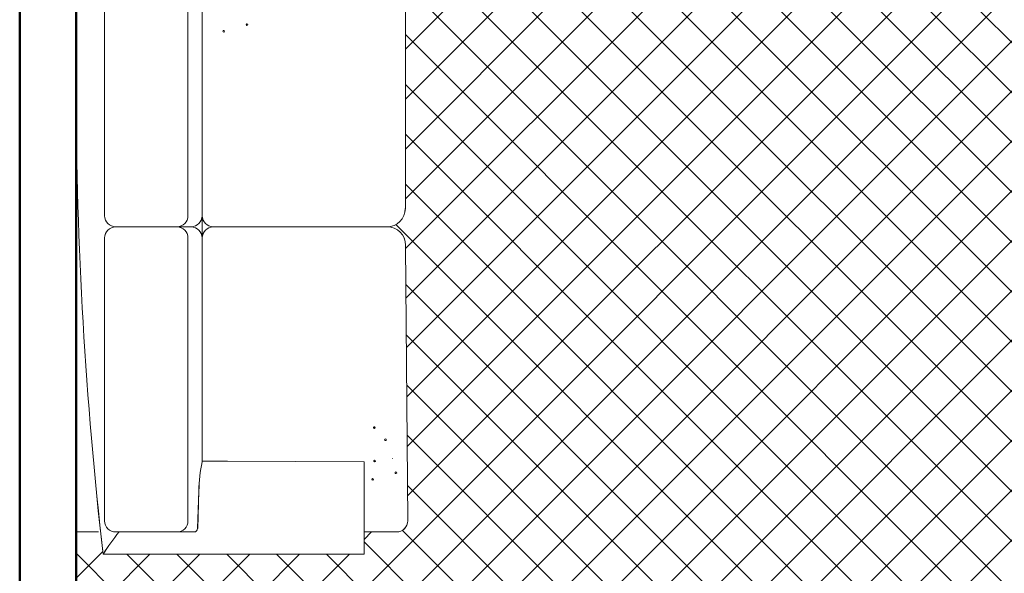
# Model space of a CAD drawing. Units: inches. Extents: x -466983 to 1020, y 324 to 318697.
# Tile 49 of 97: x 609 to 679, y 885 to 924. Entities that reach past the tile are written whole.
import ezdxf

# ---------------------------------------------------------------- set-up
doc = ezdxf.new("R2010")
doc.units = ezdxf.units.IN
doc.header["$MEASUREMENT"] = 0
for name, color, linetype, lineweight in [('A-FLOR-PATT', 252, 'Continuous', 13), ('A-FURN', 8, 'Continuous', 18), ('A-WALL', 7, 'Continuous', 50)]:
    doc.layers.add(name, color=color, linetype=linetype, lineweight=lineweight)

# ---------------------------------------------------------------- blocks, each defined once
blk = doc.blocks.new('L Shaped Sofa')
at = {"ltscale": 2}
for p, q in [((2438.01, 846.52), (2438.01, 834.58)), ((2471.77, 846.52), (2438.01, 846.52)), ((2438.01, 843.66), (2433.8, 843.66)), ((2459.54, 843.19), (2459.37, 838.32)), ((2460.02, 843.66), (2462.23, 843.66)), ((2470.14, 843.66), (2462.23, 843.66)), ((2475.26, 843.66), (2472.36, 843.66)), ((2475.26, 843.66), (2475.26, 821.69)), ((2432.65, 806.57), (2432.37, 842.21)), ((2460.8, 842.22), (2460.8, 821.69)), ((2471.57, 842.22), (2471.57, 821.69)), ((2455.69, 834.49), (2438.01, 834.58)), ((2455.69, 834.49), (2458.96, 834.49)), ((2458.96, 834.58), (2458.96, 805.64)), ((2460.8, 805.64), (2460.8, 821.69)), ((2471.57, 805.64), (2471.57, 821.69)), ((2475.26, 723.23), (2475.26, 821.69)), ((2458.96, 802.77), (2458.96, 805.64)), ((2435.07, 804.21), (2435.04, 804.21)), ((2457.53, 804.21), (2435.07, 804.21)), ((2457.53, 804.21), (2457.53, 804.21)), ((2462.23, 804.21), (2460.39, 804.21)), ((2470.14, 804.21), (2462.23, 804.21)), ((2458.96, 739.53), (2458.96, 802.77)), ((2460.8, 737.69), (2460.8, 802.77)), ((2471.57, 769.96), (2471.57, 802.77)), ((2432.68, 769.96), (2432.68, 801.82))]:
    blk.add_line(p, q, dxfattribs=at)
for centre, radius, start, end in [((2441.54, 866.11), 36.02, 321.4328, 327.0519), ((1939.08, 785.44), 536.19, 353.6823, 6.5416), ((2433.8, 842.22), 1.43, 90, 180.4579), ((2460.02, 843.18), 0.478, 90, 177.9816), ((2462.23, 842.22), 1.43, 90, 180), ((2470.14, 842.22), 1.43, 0, 90), ((2441.72, 838.37), 17.66, 347.6131, 359.8582), ((2436.91, 836.86), 0.106, 1.3946, 181.3946), ((2436.91, 836.86), 0.106, 181.3946, 1.3946), ((2433.9, 836), 0.106, 1.3946, 181.3946), ((2433.9, 836), 0.106, 181.3946, 1.3946), ((2434.34, 834.18), 0.0177, 1.3946, 181.3946), ((2434.34, 834.18), 0.0177, 181.3946, 1.3946), ((2436.66, 834.49), 0.106, 1.3946, 181.3946), ((2436.66, 834.49), 0.106, 181.3946, 1.3946), ((2435.25, 831.74), 0.106, 1.3946, 181.3946), ((2435.25, 831.74), 0.106, 181.3946, 1.3946), ((2436.69, 830.17), 0.106, 1.3946, 181.3946), ((2436.69, 830.17), 0.106, 181.3946, 1.3946), ((2435.04, 806.59), 2.39, 180.4579, 270), ((2457.53, 805.64), 1.43, 270, 0), ((2460.39, 805.64), 1.43, 180, 270), ((2462.23, 805.64), 1.43, 180, 270), ((2470.14, 805.64), 1.43, 270, 0), ((2435.07, 801.82), 2.39, 90, 180), ((2457.53, 802.77), 1.43, 0, 90), ((2460.39, 802.77), 1.43, 90, 180), ((2462.23, 802.77), 1.43, 90, 180), ((2470.14, 802.77), 1.43, 0, 90), ((2453.17, 778.06), 0.106, 1.3946, 181.3946), ((2456.17, 778.91), 0.106, 1.3946, 181.3946), ((2456.17, 778.91), 0.106, 181.3946, 1.3946), ((2453.17, 778.06), 0.106, 181.3946, 1.3946)]:
    blk.add_arc(centre, radius, start, end, dxfattribs=at)

msp = doc.modelspace()

# ---------------------------------------------------------------- hatches: boundary and pattern name
at = {"layer": 'A-FLOR-PATT', "transparency": 33554572}
h = msp.add_hatch(dxfattribs=at)
h.set_pattern_fill('ANSI37', color=256, scale=30)
h.set_pattern_definition([(45, (-1212.4137, -290.035), (-2.6516504, 2.6516504), []), (135, (-1212.4137, -290.035), (-2.6516504, -2.6516504), [])])
h.paths.add_polyline_path([(901.806, 1075.938), (900.614, 1075.938), (900.614, 1065.386), (899.391, 1065.386), (898.091, 1065.386), (892.836, 1058.71, -0.258377), (892.188, 1058.351), (879.985, 1058.351, -0.20177), (879.438, 1058.581), (874.081, 1065.386), (872.781, 1065.386), (871.558, 1065.386), (871.558, 1075.938), (813.806, 1075.938), (813.806, 1044.792), (832.395, 1044.792, -0.394795), (848.66, 1028.536), (848.66, 1009.938), (901.806, 1009.938), (901.806, 1015.938), (901.306, 1015.938), (871.306, 1015.938), (871.306, 1017.25), (871.334, 1017.25, -0.401453), (901.306, 1045.938), (901.806, 1045.938)])
edge = h.paths.add_edge_path(flags=16)
edge.add_line((847.773, 1068.949), (847.773, 1073.709))
edge.add_arc((849.227, 1073.709), 1.454, 90, 180, ccw=False)
edge.add_line((849.227, 1075.163), (864.492, 1075.163))
edge.add_arc((864.492, 1073.709), 1.454, 0, 90, ccw=False)
edge.add_line((865.946, 1073.709), (865.946, 1069.004))
edge.add_arc((832.645, 1068.976), 33.301, -20.61234, 0.04725, ccw=False)
edge.add_ellipse((856.859, 1058.48), major_axis=(0, 10.213), ratio=0.685919, start_angle=100.00884, end_angle=259.99116, ccw=False)
edge.add_arc((881.074, 1068.976), 33.301, 180.04725, 200.61234, ccw=False)
h.paths.add_polyline_path([(853.146, 1066.482), (853.146, 1066.453), (853.146, 1066.453, 0.433107), (852.917, 1066.685), (852.917, 1066.453), (853.146, 1066.453), (853.146, 1066.482), (853.088, 1066.612, 0.697939), (852.7, 1066.453), (852.7, 1066.453), (852.7, 1066.482), (852.917, 1067.001), (852.917, 1066.685, -0.396254)], flags=0)
h.paths.add_polyline_path([(861.019, 1066.482), (861.019, 1066.453), (861.019, 1066.453, 0.416404), (860.802, 1066.685), (860.802, 1066.453), (861.019, 1066.453), (861.019, 1066.482), (860.967, 1066.605, 0.713344), (860.573, 1066.453), (860.573, 1066.453), (860.573, 1066.482), (860.802, 1067.001), (860.802, 1066.685, -0.379973)], flags=0)
edge = h.paths.add_edge_path(flags=0)
edge.add_spline(control_points=[(861.13, 1065.785), (861.466, 1065.248), (861.613, 1065.016), (861.983, 1064.374), (862.192, 1063.944), (862.561, 1063.039), (862.721, 1062.563), (862.987, 1061.578), (863.092, 1061.069), (863.245, 1060.031), (863.293, 1059.503), (863.329, 1058.441), (863.318, 1057.908), (863.237, 1056.852), (863.166, 1056.329), (862.97, 1055.308), (862.843, 1054.81), (862.537, 1053.852), (862.357, 1053.393), (861.951, 1052.525), (861.725, 1052.117), (861.233, 1051.362), (860.967, 1051.016), (860.405, 1050.395), (860.108, 1050.12), (859.494, 1049.646), (859.176, 1049.448), (858.528, 1049.13), (858.197, 1049.011), (857.531, 1048.852), (857.196, 1048.812), (856.525, 1048.812), (856.189, 1048.852), (855.524, 1049.01), (855.193, 1049.129), (854.545, 1049.447), (854.227, 1049.645), (853.612, 1050.118), (853.316, 1050.393), (852.753, 1051.014), (852.487, 1051.36), (851.995, 1052.114), (851.769, 1052.523), (851.363, 1053.39), (851.183, 1053.85), (850.877, 1054.807), (850.75, 1055.305), (850.553, 1056.326), (850.483, 1056.849), (850.401, 1057.905), (850.39, 1058.438), (850.426, 1059.5), (850.473, 1060.028), (850.626, 1061.066), (850.732, 1061.575), (850.997, 1062.561), (851.157, 1063.036), (851.525, 1063.942), (851.734, 1064.371), (852.106, 1065.016), (852.254, 1065.25), (852.608, 1065.733)], knot_values=[3.915332, 3.915332, 3.915332, 3.915332, 4.013468, 4.013468, 4.175532, 4.175532, 4.337596, 4.337596, 4.49966, 4.49966, 4.661724, 4.661724, 4.823788, 4.823788, 4.985852, 4.985852, 5.147916, 5.147916, 5.30998, 5.30998, 5.472044, 5.472044, 5.634109, 5.634109, 5.796173, 5.796173, 5.958237, 5.958237, 6.120301, 6.120301, 6.282365, 6.282365, 6.444429, 6.444429, 6.606493, 6.606493, 6.768557, 6.768557, 6.930621, 6.930621, 7.092685, 7.092685, 7.254749, 7.254749, 7.416813, 7.416813, 7.578878, 7.578878, 7.740942, 7.740942, 7.903006, 7.903006, 8.06507, 8.06507, 8.227134, 8.227134, 8.389198, 8.389198, 8.551262, 8.551262, 8.65037, 8.65037, 8.65037, 8.65037], degree=3, periodic=0)
edge.add_line((852.642, 1065.785), (861.13, 1065.785))
edge = h.paths.add_edge_path(flags=0)
edge.add_ellipse((856.85, 1057.743), major_axis=(0, 7.792), ratio=0.687861, start_angle=0, end_angle=360)
h.paths.add_polyline_path([(848.863, 1069.389), (848.863, 1073.96, -0.414214), (849.954, 1075.051), (863.765, 1075.051, -0.414214), (864.856, 1073.96), (864.856, 1069.389, -0.388936), (864.524, 1069.027, -0.043561), (849.195, 1069.027, -0.388936)], flags=0)
h.paths.add_polyline_path([(853.101, 1068.112, -1), (852.677, 1068.112, -1)], flags=0)
edge = h.paths.add_edge_path(flags=0)
edge.add_ellipse((856.859, 1057.338), major_axis=(0, 2.207), ratio=0.657164, start_angle=0, end_angle=360)
h.paths.add_polyline_path([(861.041, 1068.112, -1), (860.618, 1068.112, -1)], flags=0)
edge = h.paths.add_edge_path()
edge.add_line((573.954, 1057.341), (573.954, 1075.938))
edge.add_line((573.954, 1075.938), (558.731, 1075.938))
edge.add_line((558.731, 1075.938), (558.731, 1065.386))
edge.add_line((558.731, 1065.386), (557.507, 1065.386))
edge.add_line((557.507, 1065.386), (556.207, 1065.386))
edge.add_line((556.207, 1065.386), (550.952, 1058.71))
edge.add_arc((550.304, 1059.116), 0.765, 270, 327.94832, ccw=False)
edge.add_line((550.304, 1058.351), (538.101, 1058.351))
edge.add_arc((538.101, 1059.116), 0.765, 224.3704, 270, ccw=False)
edge.add_line((537.555, 1058.581), (532.198, 1065.386))
edge.add_line((532.198, 1065.386), (530.898, 1065.386))
edge.add_line((530.898, 1065.386), (529.674, 1065.386))
edge.add_line((529.674, 1065.386), (529.674, 1075.938))
edge.add_line((529.674, 1075.938), (520.806, 1075.938))
edge.add_line((520.806, 1075.938), (520.806, 1045.938))
edge.add_line((520.806, 1045.938), (521.306, 1045.938))
edge.add_arc((521.306, 1015.938), 30, 2.50749, 90, ccw=False)
edge.add_line((551.277, 1017.25), (551.306, 1017.25))
edge.add_line((551.306, 1017.25), (551.306, 1015.938))
edge.add_line((551.306, 1015.938), (520.806, 1015.938))
edge.add_line((520.806, 1015.938), (520.806, 1009.938))
edge.add_line((520.806, 1009.938), (559.191, 1010.402))
edge.add_arc((559.191, 1011.856), 1.454, 180, 270, ccw=False)
edge.add_line((557.737, 1011.856), (557.737, 1016.561))
edge.add_arc((591.039, 1016.589), 33.301, 159.38766, 180.04725, ccw=False)
edge.add_ellipse((566.824, 1027.085), major_axis=(0, 10.213), ratio=0.685919, start_angle=280.00884, end_angle=439.99116, ccw=False)
edge.add_arc((542.609, 1016.589), 33.301, 0.04725, 20.61234, ccw=False)
edge.add_line((575.91, 1016.616), (575.91, 1011.856))
edge.add_arc((574.456, 1011.856), 1.454, -90, 0, ccw=False)
edge.add_line((574.456, 1010.402), (608.806, 1009.938))
edge.add_line((608.806, 1009.938), (608.806, 1041.086))
edge.add_line((608.806, 1041.086), (590.218, 1041.086))
edge.add_arc((590.775, 1057.907), 16.831, 181.92775, 268.10321, ccw=False)
edge = h.paths.add_edge_path()
edge.add_ellipse((494.244, 583.62), major_axis=(0, 10.213), ratio=0.685919, start_angle=280.00884, end_angle=439.99116, ccw=False)
edge.add_arc((470.03, 573.124), 33.301, 0.04725, 20.61234, ccw=False)
edge.add_line((503.331, 573.152), (503.331, 568.392))
edge.add_arc((501.877, 568.392), 1.454, -90, 0, ccw=False)
edge.add_line((501.877, 566.938), (539.806, 566.938))
edge.add_line((539.806, 566.938), (539.806, 572.938))
edge.add_line((539.806, 572.938), (539.306, 572.938))
edge.add_line((539.306, 572.938), (509.306, 572.938))
edge.add_line((509.306, 572.938), (509.306, 574.25))
edge.add_line((509.306, 574.25), (509.334, 574.25))
edge.add_arc((539.306, 572.938), 30, 90, 177.49251, ccw=False)
edge.add_line((539.306, 602.938), (539.806, 602.938))
edge.add_line((539.806, 602.938), (539.806, 626.938))
edge.add_line((539.806, 626.938), (531.772, 626.938))
edge.add_line((531.772, 626.938), (531.772, 616.386))
edge.add_line((531.772, 616.386), (530.548, 616.386))
edge.add_line((530.548, 616.386), (529.249, 616.386))
edge.add_line((529.249, 616.386), (523.711, 609.351))
edge.add_line((523.711, 609.351), (510.777, 609.351))
edge.add_line((510.777, 609.351), (505.239, 616.386))
edge.add_line((505.239, 616.386), (503.939, 616.386))
edge.add_line((503.939, 616.386), (502.715, 616.386))
edge.add_line((502.715, 616.386), (502.715, 626.938))
edge.add_line((502.715, 626.938), (481.698, 626.938))
edge.add_line((481.698, 626.938), (481.698, 610.995))
edge.add_arc((467.27, 611.473), 14.436, 271.92775, 358.10321, ccw=False)
edge.add_line((467.756, 597.045), (451.806, 597.045))
edge.add_line((451.806, 597.045), (451.806, 584.404))
edge.add_line((451.806, 584.404), (451.806, 566.938))
edge.add_line((451.806, 566.938), (486.612, 566.938))
edge.add_arc((486.612, 568.392), 1.454, 180, 270, ccw=False)
edge.add_line((485.158, 568.392), (485.158, 573.097))
edge.add_arc((518.459, 573.124), 33.301, 159.38766, 180.04725, ccw=False)
h.paths.add_polyline_path([(836.261, 1020.733), (879.89, 1020.733), (879.89, 1039.39), (836.261, 1039.39)], flags=25)
h.paths.add_polyline_path([(549.985, 1036.749), (593.614, 1036.749), (593.614, 1055.407), (549.985, 1055.407)], flags=24)
h.paths.add_polyline_path([(475.123, 595.596), (518.752, 595.596), (518.752, 614.253), (475.123, 614.253)], flags=24)
h = msp.add_hatch(dxfattribs=at)
h.set_pattern_fill('ANSI37', color=256, scale=20)
h.set_pattern_definition([(45, (-1212.4137, -290.035), (-1.767767, 1.767767), []), (135, (-1212.4137, -290.035), (-1.767767, -1.767767), [])])
h.paths.add_polyline_path([(809.806, 870.938), (809.806, 888.152), (806.998, 888.152), (802.662, 888.152), (789.383, 888.152), (786.285, 888.152, -0.414214), (785.499, 888.937), (785.499, 900.196), (785.499, 908.47, -0.414214), (786.808, 909.779, -0.414214), (785.499, 911.088), (785.499, 929.101, -0.414214), (786.808, 930.411, -0.414214), (785.499, 931.72), (785.499, 931.904, -0.414214), (784.19, 930.595), (766.722, 930.595, -0.412359), (765.413, 931.896, -0.413741), (764.115, 930.578), (744.578, 930.422, -0.416556), (743.786, 931.207), (743.786, 933.515), (742.215, 933.515), (742.215, 952.024, -0.001344), (743.786, 952.2), (743.786, 953.938), (678.592, 953.938), (678.592, 951.131), (678.592, 946.794), (678.592, 933.515), (678.592, 930.417, -0.414214), (677.806, 929.631), (666.548, 929.631), (658.274, 929.631, -0.414214), (656.965, 930.94, -0.414214), (655.656, 929.631), (637.642, 929.631, -0.414214), (636.333, 930.94, -0.414214), (635.024, 929.631), (634.839, 929.631, -0.414214), (636.149, 928.322), (636.149, 910.854, -0.412359), (634.848, 909.545, -0.413741), (636.165, 908.247), (636.321, 888.71, -0.416556), (635.536, 887.918), (633.228, 887.918), (633.228, 886.347), (614.719, 886.347, -0.001344), (614.544, 887.918), (612.806, 887.918), (612.806, 834.938), (612.806, 752.938), (612.806, 748.938), (612.806, 697.938), (654.806, 697.938), (654.806, 701.938), (715.806, 701.938), (715.806, 737.435), (774.292, 737.435), (774.292, 795.938), (809.806, 795.938)])
h.paths.add_polyline_path([(679.276, 849.576, 0.102523), (682.148, 849.261, -0.080461), (694.543, 849.773, -0.283899), (694.482, 849.008, 0.136605), (694.407, 848.81, -0.030441), (694.543, 846.893), (694.543, 842.62), (694.543, 838.347, -0.028219), (694.425, 836.568), (694.425, 836.568, 0.196187), (694.446, 836.271, -0.302897), (694.543, 835.467, -0.080461), (682.148, 835.979, 0.102523), (679.276, 835.664, -0.58611), (678.646, 836.017), (678.646, 849.223, -0.58611)], flags=16)
h.paths.add_polyline_path([(679.517, 848.651, 0.699597), (679.476, 848.634, 1.20716), (679.194, 848.742, 0.010621)], flags=0)
h.paths.add_polyline_path([(679.492, 836.561, -0.013798), (679.918, 836.659, -0.071703), (682.853, 837.143, -0.165743), (682.166, 839.101), (682.166, 842.609), (682.166, 846.06, -0.240616), (683.473, 848.677, -0.068263), (693.929, 849.008), (693.788, 848.708), (693.788, 849.023, 0.067332), (683.473, 848.677, 0.240616), (682.166, 846.06), (682.166, 842.609), (682.166, 839.101, 0.23459), (683.461, 836.551, 0.068093), (693.788, 836.195), (693.788, 836.51), (693.93, 836.21, -0.077215), (682.242, 836.782, 0.086627), (679.528, 836.57, -0.628402), (679.503, 836.573), (679.503, 836.607, 0.910458)], flags=0)
h.paths.add_polyline_path([(679.476, 848.636), (679.207, 848.647), (679.207, 836.572, 0.913566), (679.365, 836.586), (679.476, 836.582)], flags=0)
h.paths.add_polyline_path([(679.276, 829.86, 0.102523), (682.148, 829.546, -0.080461), (694.543, 830.057, -0.283899), (694.482, 829.293, 0.136605), (694.407, 829.095, -0.030441), (694.543, 827.178), (694.543, 822.904), (694.543, 818.631, -0.028219), (694.425, 816.853), (694.425, 816.853, 0.196187), (694.446, 816.556, -0.302897), (694.543, 815.752, -0.080461), (682.148, 816.263, 0.102523), (679.276, 815.949, -0.58611), (678.646, 816.302), (678.646, 829.507, -0.58611)], flags=16)
h.paths.add_polyline_path([(679.517, 828.936, 0.699597), (679.476, 828.919, 1.20716), (679.194, 829.027, 0.010621)], flags=0)
h.paths.add_polyline_path([(679.492, 816.846, -0.013798), (679.918, 816.944, -0.071703), (682.853, 817.428, -0.165743), (682.166, 819.385), (682.166, 822.894), (682.166, 826.345, -0.240616), (683.473, 828.961, -0.068263), (693.929, 829.293), (693.788, 828.993), (693.788, 829.308, 0.067332), (683.473, 828.961, 0.240616), (682.166, 826.345), (682.166, 822.894), (682.166, 819.385, 0.23459), (683.461, 816.836, 0.068093), (693.788, 816.48), (693.788, 816.795), (693.93, 816.495, -0.077215), (682.242, 817.066, 0.086627), (679.528, 816.855, -0.628402), (679.503, 816.858), (679.503, 816.892, 0.910458)], flags=0)
h.paths.add_polyline_path([(679.476, 828.921), (679.207, 828.932), (679.207, 816.857, 0.913566), (679.365, 816.871), (679.476, 816.867)], flags=0)
h.paths.add_polyline_path([(679.276, 810.145, 0.102523), (682.148, 809.83, -0.080461), (694.543, 810.342, -0.3023), (694.447, 809.539, 0.10023), (694.406, 809.388, -0.03057), (694.543, 807.462), (694.543, 803.189), (694.543, 798.916, -0.03057), (694.406, 796.991, 0.10023), (694.447, 796.839, -0.3023), (694.543, 796.036, -0.080461), (682.148, 796.548, 0.102523), (679.276, 796.233, -0.58611), (678.646, 796.586), (678.646, 809.792, -0.58611)], flags=16)
h.paths.add_polyline_path([(679.517, 809.242, 0.699597), (679.476, 809.224, 1.20716), (679.194, 809.332, 0.010621)], flags=0)
h.paths.add_polyline_path([(679.492, 797.151, -0.013798), (679.918, 797.25, -0.071703), (682.853, 797.734, -0.165743), (682.166, 799.691), (682.166, 803.2), (682.166, 806.65, -0.239349), (683.461, 809.258, -0.072465), (694.447, 809.541, 0.197932), (694.425, 809.241), (693.788, 809.299), (693.788, 809.614, 0.068093), (683.461, 809.258, 0.239349), (682.166, 806.65), (682.166, 803.2), (682.166, 799.691, 0.235854), (683.473, 797.132, 0.067332), (693.788, 796.786), (693.788, 797.101), (694.425, 797.159, 0.197932), (694.447, 796.859, -0.080419), (682.156, 797.379, 0.083867), (679.528, 797.16, -0.628402), (679.503, 797.164), (679.503, 797.197, 0.910458)], flags=0)
h.paths.add_polyline_path([(679.207, 809.237), (679.207, 797.162, 0.913566), (679.365, 797.176), (679.476, 797.173), (679.476, 809.227)], flags=0)
h.paths.add_polyline_path([(695.364, 853.299), (728.223, 853.299), (728.223, 771.152), (695.364, 771.152)], flags=16)
h.paths.add_polyline_path([(696.021, 852.642), (727.566, 852.642), (727.566, 771.809), (696.021, 771.809)], flags=0)
h.paths.add_polyline_path([(679.276, 788.787, 0.102523), (682.148, 788.472, -0.080461), (694.543, 788.984, -0.3023), (694.447, 788.181, 0.10023), (694.406, 788.03, -0.03057), (694.543, 786.104), (694.543, 781.831), (694.543, 777.558, -0.03057), (694.406, 775.632, 0.10023), (694.447, 775.481, -0.3023), (694.543, 774.678, -0.080461), (682.148, 775.19, 0.102523), (679.276, 774.875, -0.58611), (678.646, 775.228), (678.646, 788.434, -0.58611)], flags=16)
h.paths.add_polyline_path([(679.517, 787.883, 0.699597), (679.476, 787.866, 1.20716), (679.194, 787.974, 0.010621)], flags=0)
h.paths.add_polyline_path([(679.492, 775.793, -0.013798), (679.918, 775.891, -0.071703), (682.853, 776.375, -0.165743), (682.166, 778.333), (682.166, 781.841), (682.166, 785.292, -0.239349), (683.461, 787.899, -0.072465), (694.447, 788.182, 0.197932), (694.425, 787.882), (693.788, 787.94), (693.788, 788.255, 0.068093), (683.461, 787.899, 0.239349), (682.166, 785.292), (682.166, 781.841), (682.166, 778.333, 0.235854), (683.473, 775.774, 0.067332), (693.788, 775.428), (693.788, 775.742), (694.425, 775.8, 0.197932), (694.447, 775.5, -0.080419), (682.156, 776.021, 0.083867), (679.528, 775.802, -0.628402), (679.503, 775.805), (679.503, 775.839, 0.910458)], flags=0)
h.paths.add_polyline_path([(679.207, 787.879), (679.207, 775.804, 0.913566), (679.365, 775.818), (679.476, 775.814), (679.476, 787.868)], flags=0)
h.paths.add_polyline_path([(704.641, 854.12, -0.080461), (705.153, 866.516, 0.102523), (704.838, 869.387, -0.58611), (705.191, 870.017), (718.397, 870.017, -0.58611), (718.75, 869.387, 0.102523), (718.435, 866.516, -0.080461), (718.946, 854.12, -0.3023), (718.144, 854.217, 0.10023), (717.992, 854.257, -0.03057), (716.067, 854.12), (711.794, 854.12), (707.521, 854.12, -0.03057), (705.595, 854.257, 0.10023), (705.444, 854.217, -0.3023)], flags=16)
h.paths.add_polyline_path([(717.846, 869.146, 0.699597), (717.829, 869.187, 1.20716), (717.937, 869.47, 0.010621)], flags=0)
h.paths.add_polyline_path([(705.463, 854.216, -0.080419), (705.984, 866.507, 0.083867), (705.765, 869.135, -0.628402), (705.768, 869.16), (705.802, 869.16, 0.910458), (705.756, 869.171, -0.013798), (705.854, 868.745, -0.071703), (706.338, 865.81, -0.165743), (708.295, 866.497), (711.804, 866.497), (715.255, 866.497, -0.239349), (717.862, 865.202, -0.072465), (718.145, 854.216, 0.197932), (717.845, 854.238), (717.903, 854.876), (718.218, 854.876, 0.068093), (717.862, 865.202, 0.239349), (715.255, 866.497), (711.804, 866.497), (708.295, 866.497, 0.235854), (705.737, 865.19, 0.067332), (705.391, 854.876), (705.705, 854.876), (705.763, 854.238, 0.197932)], flags=16)
h.paths.add_polyline_path([(705.766, 869.456, 0.913566), (705.781, 869.299), (705.777, 869.187), (717.831, 869.187), (717.842, 869.456)], flags=0)
h.paths.add_polyline_path([(729.045, 842.62), (729.045, 846.893, -0.03057), (729.182, 848.818, 0.10023), (729.141, 848.97, -0.3023), (729.045, 849.773, -0.080461), (741.44, 849.261, 0.102523), (744.311, 849.576, -0.58611), (744.942, 849.223), (744.942, 836.017, -0.58611), (744.311, 835.664, 0.102523), (741.44, 835.979, -0.080461), (729.045, 835.467, -0.3023), (729.141, 836.27, 0.10023), (729.182, 836.421, -0.03057), (729.045, 838.347)], flags=16)
h.paths.add_polyline_path([(744.111, 836.585, 1.20716), (744.394, 836.477, 0.010621), (744.07, 836.567, 0.699597)], flags=0)
h.paths.add_polyline_path([(729.141, 836.268, 0.197932), (729.162, 836.568), (729.8, 836.51), (729.8, 836.195, 0.068093), (740.126, 836.551, 0.239349), (741.421, 839.159), (741.421, 842.609), (741.421, 846.118, 0.235854), (740.114, 848.677, 0.067332), (729.8, 849.023), (729.8, 848.708), (729.162, 848.65, 0.197932), (729.141, 848.95, -0.080419), (741.432, 848.43, 0.083867), (744.059, 848.649, -0.628402), (744.085, 848.645), (744.085, 848.612, 0.910458), (744.095, 848.658, -0.013798), (743.67, 848.559, -0.071703), (740.734, 848.075, -0.165743), (741.421, 846.118), (741.421, 842.609), (741.421, 839.159, -0.239349), (740.126, 836.551, -0.072465)], flags=0)
h.paths.add_polyline_path([(729.045, 830.057, -0.080461), (741.44, 829.546, 0.102523), (744.311, 829.86, -0.58611), (744.942, 829.507), (744.942, 816.302, -0.58611), (744.311, 815.949, 0.102523), (741.44, 816.263, -0.080461), (729.045, 815.752, -0.3023), (729.141, 816.554, 0.10023), (729.182, 816.706, -0.03057), (729.045, 818.631), (729.045, 822.904), (729.045, 827.178, -0.03057), (729.182, 829.103, 0.10023), (729.141, 829.255, -0.3023)], flags=16)
h.paths.add_polyline_path([(744.111, 816.869, 1.20716), (744.394, 816.761, 0.010621), (744.07, 816.852, 0.699597)], flags=0)
h.paths.add_polyline_path([(729.141, 829.235, -0.080419), (741.432, 828.714, 0.083867), (744.059, 828.933, -0.628402), (744.085, 828.93), (744.085, 828.896, 0.910458), (744.095, 828.943, -0.013798), (743.67, 828.844, -0.071703), (740.734, 828.36, -0.165743), (741.421, 826.403), (741.421, 822.894), (741.421, 819.443, -0.239349), (740.126, 816.836, -0.072465), (729.141, 816.553, 0.197932), (729.162, 816.853), (729.8, 816.795), (729.8, 816.48, 0.068093), (740.126, 816.836, 0.239349), (741.421, 819.443), (741.421, 822.894), (741.421, 826.403, 0.235854), (740.114, 828.961, 0.067332), (729.8, 829.308), (729.8, 828.993), (729.162, 828.935, 0.197932)], flags=16)
h.paths.add_polyline_path([(729.045, 810.342, -0.080461), (741.44, 809.83, 0.102523), (744.311, 810.145, -0.58611), (744.942, 809.792), (744.942, 796.586, -0.58611), (744.311, 796.233, 0.102523), (741.44, 796.548, -0.080461), (729.045, 796.036, -0.283899), (729.105, 796.801, 0.136605), (729.181, 796.999, -0.030441), (729.045, 798.916), (729.045, 803.189), (729.045, 807.462, -0.028219), (729.163, 809.241), (729.162, 809.241, 0.196187), (729.142, 809.538, -0.302897)], flags=16)
h.paths.add_polyline_path([(744.111, 797.175, 1.20716), (744.394, 797.067, 0.010621), (744.07, 797.158, 0.699597)], flags=0)
h.paths.add_polyline_path([(741.345, 809.027, 0.086627), (744.059, 809.239, -0.628402), (744.085, 809.235), (744.085, 809.202, 0.910458), (744.095, 809.248, -0.013798), (743.67, 809.15, -0.071703), (740.734, 808.666, -0.165743), (741.421, 806.708), (741.421, 803.2), (741.421, 799.749, -0.240616), (740.114, 797.132, -0.068263), (729.658, 796.801), (729.8, 797.101), (729.8, 796.786, 0.067332), (740.114, 797.132, 0.240616), (741.421, 799.749), (741.421, 803.2), (741.421, 806.708, 0.23459), (740.126, 809.258, 0.068093), (729.8, 809.614), (729.8, 809.299), (729.658, 809.599, -0.077215)], flags=0)
h.paths.add_polyline_path([(704.641, 770.33, -0.283899), (705.405, 770.27, 0.136605), (705.603, 770.194, -0.030441), (707.521, 770.33), (711.794, 770.33), (716.067, 770.33, -0.028219), (717.845, 770.212), (717.845, 770.213, 0.196187), (718.143, 770.233, -0.302897), (718.946, 770.33, -0.080461), (718.435, 757.935, 0.102523), (718.75, 755.064, -0.58611), (718.397, 754.433), (705.191, 754.433, -0.58611), (704.838, 755.064, 0.102523), (705.153, 757.935, -0.080461)], flags=16)
h.paths.add_polyline_path([(705.762, 755.305, 0.699597), (705.779, 755.264, 1.20716), (705.671, 754.981, 0.010621)], flags=0)
h.paths.add_polyline_path([(705.405, 769.717), (705.705, 769.575), (705.391, 769.575, 0.067332), (705.737, 759.261, 0.240616), (708.353, 757.954), (711.804, 757.954), (715.313, 757.954, 0.23459), (717.862, 759.249, 0.068093), (718.218, 769.575), (717.903, 769.575), (718.203, 769.717, -0.077215), (717.632, 758.03, 0.086627), (717.843, 755.316, -0.628402), (717.84, 755.29), (717.806, 755.29, 0.910458), (717.853, 755.28, -0.013798), (717.754, 755.705, -0.071703), (717.27, 758.641, -0.165743), (715.313, 757.954), (711.804, 757.954), (708.353, 757.954, -0.240616), (705.737, 759.261, -0.068263)], flags=0)
h.paths.add_polyline_path([(729.045, 788.984, -0.080461), (741.44, 788.472, 0.102523), (744.311, 788.787, -0.58611), (744.942, 788.434), (744.942, 775.228, -0.58611), (744.311, 774.875, 0.102523), (741.44, 775.19, -0.080461), (729.045, 774.678, -0.283899), (729.105, 775.443, 0.136605), (729.181, 775.64, -0.030441), (729.045, 777.558), (729.045, 781.831), (729.045, 786.104, -0.028219), (729.163, 787.882), (729.162, 787.882, 0.196187), (729.142, 788.18, -0.302897)], flags=16)
h.paths.add_polyline_path([(744.111, 775.817, 1.20716), (744.394, 775.709, 0.010621), (744.07, 775.799, 0.699597)], flags=0)
h.paths.add_polyline_path([(741.345, 787.669, 0.086627), (744.059, 787.881, -0.628402), (744.085, 787.877), (744.085, 787.844, 0.910458), (744.095, 787.89, -0.013798), (743.67, 787.791, -0.071703), (740.734, 787.307, -0.165743), (741.421, 785.35), (741.421, 781.841), (741.421, 778.39, -0.240616), (740.114, 775.774, -0.068263), (729.658, 775.443), (729.8, 775.742), (729.8, 775.428, 0.067332), (740.114, 775.774, 0.240616), (741.421, 778.39), (741.421, 781.841), (741.421, 785.35, 0.23459), (740.126, 787.899, 0.068093), (729.8, 788.255), (729.8, 787.94), (729.658, 788.241, -0.077215)], flags=0)
h.paths.add_polyline_path([(744.111, 848.636), (744.111, 836.582), (744.381, 836.572), (744.381, 848.647, 0.913566), (744.223, 848.633)], flags=0)
h.paths.add_polyline_path([(744.223, 828.917), (744.111, 828.921), (744.111, 816.867), (744.381, 816.857), (744.381, 828.932, 0.913566)], flags=0)
h.paths.add_polyline_path([(717.831, 755.264), (705.777, 755.264), (705.766, 754.994), (717.842, 754.994, 0.913566), (717.827, 755.152)], flags=0)
h.paths.add_polyline_path([(744.223, 809.223), (744.111, 809.227), (744.111, 797.173), (744.381, 797.162), (744.381, 809.237, 0.913566)], flags=0)
h.paths.add_polyline_path([(744.111, 787.868), (744.111, 775.814), (744.381, 775.804), (744.381, 787.879, 0.913566), (744.223, 787.865)], flags=0)
h.paths.add_polyline_path([(678.877, 877.123), (737.613, 877.123), (737.613, 899.512), (678.877, 899.512)], flags=24)

# ---------------------------------------------------------------- linework, layer by layer
at = {"layer": 'A-FURN', "ltscale": 2}
for p, q in [((612.806, 953.938), (612.806, 899.962)), ((612.806, 953.938), (612.806, 899.962)), ((612.806, 953.938), (612.806, 899.962)), ((612.806, 953.938), (612.806, 899.962)), ((612.806, 953.938), (612.806, 899.962)), ((612.806, 953.938), (612.806, 899.962)), ((620.734, 946.009), (620.734, 910.331)), ((620.734, 946.009), (620.734, 910.331)), ((620.734, 946.009), (620.734, 910.331)), ((620.734, 946.009), (620.734, 910.331)), ((620.734, 946.009), (620.734, 910.331)), ((620.734, 946.009), (620.734, 910.331)), ((621.743, 945), (621.743, 910.331)), ((621.743, 945), (621.743, 910.331)), ((621.743, 945), (621.743, 910.331)), ((621.743, 945), (621.743, 910.331)), ((621.743, 945), (621.743, 910.331)), ((621.743, 945), (621.743, 910.331)), ((614.827, 928.322), (614.827, 910.331)), ((614.827, 928.322), (614.827, 910.331)), ((614.827, 928.322), (614.827, 910.331)), ((614.827, 928.322), (614.827, 910.331)), ((614.827, 928.322), (614.827, 910.331)), ((614.827, 928.322), (614.827, 910.331)), ((636.149, 928.322), (636.149, 910.854)), ((636.149, 928.322), (636.149, 910.854)), ((636.149, 928.322), (636.149, 910.854)), ((636.149, 928.322), (636.149, 910.854)), ((636.149, 928.322), (636.149, 910.854)), ((636.149, 928.322), (636.149, 910.854)), ((621.743, 910.331), (621.743, 908.76)), ((621.743, 910.331), (621.743, 908.76)), ((621.743, 910.331), (621.743, 908.76)), ((621.743, 910.331), (621.743, 908.76)), ((621.743, 910.331), (621.743, 908.76)), ((621.743, 910.331), (621.743, 908.76)), ((615.613, 909.545), (619.949, 909.545)), ((615.613, 909.545), (619.949, 909.545)), ((615.613, 909.545), (619.949, 909.545)), ((615.613, 909.545), (619.949, 909.545)), ((615.613, 909.545), (619.949, 909.545)), ((615.613, 909.545), (619.949, 909.545)), ((619.949, 909.545), (620.958, 909.545)), ((619.949, 909.545), (620.958, 909.545)), ((619.949, 909.545), (620.958, 909.545)), ((619.949, 909.545), (620.958, 909.545)), ((619.949, 909.545), (620.958, 909.545)), ((619.949, 909.545), (620.958, 909.545)), ((622.529, 909.545), (622.529, 909.545)), ((622.529, 909.545), (634.839, 909.545)), ((622.529, 909.545), (622.529, 909.545)), ((622.529, 909.545), (634.839, 909.545)), ((622.529, 909.545), (622.529, 909.545)), ((622.529, 909.545), (634.839, 909.545)), ((622.529, 909.545), (622.529, 909.545)), ((622.529, 909.545), (634.839, 909.545)), ((622.529, 909.545), (622.529, 909.545)), ((622.529, 909.545), (634.839, 909.545)), ((622.529, 909.545), (622.529, 909.545)), ((622.529, 909.545), (634.839, 909.545)), ((634.839, 909.545), (634.856, 909.545)), ((634.839, 909.545), (634.856, 909.545)), ((634.839, 909.545), (634.856, 909.545)), ((634.839, 909.545), (634.856, 909.545)), ((634.839, 909.545), (634.856, 909.545)), ((634.839, 909.545), (634.856, 909.545)), ((614.827, 908.76), (614.827, 899.962)), ((614.827, 908.76), (614.827, 899.962)), ((614.827, 908.76), (614.827, 899.962)), ((614.827, 908.76), (614.827, 899.962)), ((614.827, 908.76), (614.827, 899.962)), ((614.827, 908.76), (614.827, 899.962)), ((620.734, 908.76), (620.734, 899.962)), ((620.734, 908.76), (620.734, 899.962)), ((620.734, 908.76), (620.734, 899.962)), ((620.734, 908.76), (620.734, 899.962)), ((620.734, 908.76), (620.734, 899.962)), ((620.734, 908.76), (620.734, 899.962)), ((621.743, 892.893), (621.743, 908.76)), ((621.743, 892.893), (621.743, 908.76)), ((621.743, 892.893), (621.743, 908.76)), ((621.743, 892.893), (621.743, 908.76)), ((621.743, 892.893), (621.743, 908.76)), ((621.743, 892.893), (621.743, 908.76)), ((636.165, 908.247), (636.321, 888.71)), ((636.165, 908.247), (636.321, 888.71)), ((636.165, 908.247), (636.321, 888.71)), ((636.165, 908.247), (636.321, 888.71)), ((636.165, 908.247), (636.321, 888.71)), ((636.165, 908.247), (636.321, 888.71)), ((612.806, 887.918), (612.806, 899.962)), ((612.806, 887.918), (612.806, 899.962)), ((612.806, 887.918), (612.806, 899.962)), ((612.806, 887.918), (612.806, 899.962)), ((612.806, 887.918), (612.806, 899.962)), ((612.806, 887.918), (612.806, 899.962)), ((614.827, 888.704), (614.827, 899.962)), ((614.827, 888.704), (614.827, 899.962)), ((614.827, 888.704), (614.827, 899.962)), ((614.827, 888.704), (614.827, 899.962)), ((614.827, 888.704), (614.827, 899.962)), ((614.827, 888.704), (614.827, 899.962)), ((620.734, 888.704), (620.734, 899.962)), ((620.734, 888.704), (620.734, 899.962)), ((620.734, 888.704), (620.734, 899.962)), ((620.734, 888.704), (620.734, 899.962)), ((620.734, 888.704), (620.734, 899.962)), ((620.734, 888.704), (620.734, 899.962)), ((623.535, 892.943), (621.743, 892.943)), ((623.535, 892.943), (621.743, 892.943)), ((623.535, 892.943), (621.743, 892.943)), ((623.535, 892.943), (621.743, 892.943)), ((623.535, 892.943), (621.743, 892.943)), ((623.535, 892.943), (621.743, 892.943)), ((623.535, 892.943), (633.228, 892.893)), ((623.535, 892.943), (633.228, 892.893)), ((623.535, 892.943), (633.228, 892.893)), ((623.535, 892.943), (633.228, 892.893)), ((623.535, 892.943), (633.228, 892.893)), ((623.535, 892.943), (633.228, 892.893)), ((633.228, 886.347), (633.228, 892.893)), ((633.228, 886.347), (633.228, 892.893)), ((633.228, 886.347), (633.228, 892.893)), ((633.228, 886.347), (633.228, 892.893)), ((633.228, 886.347), (633.228, 892.893)), ((633.228, 886.347), (633.228, 892.893)), ((621.424, 888.171), (621.518, 890.841)), ((621.424, 888.171), (621.518, 890.841)), ((621.424, 888.171), (621.518, 890.841)), ((621.424, 888.171), (621.518, 890.841)), ((621.424, 888.171), (621.518, 890.841)), ((621.424, 888.171), (621.518, 890.841)), ((612.806, 887.918), (614.395, 887.918)), ((612.806, 887.918), (614.395, 887.918)), ((612.806, 887.918), (614.395, 887.918)), ((612.806, 887.918), (614.395, 887.918)), ((612.806, 887.918), (614.395, 887.918)), ((612.806, 887.918), (614.395, 887.918)), ((615.613, 887.918), (619.949, 887.918)), ((615.613, 887.918), (619.949, 887.918)), ((615.613, 887.918), (619.949, 887.918)), ((615.613, 887.918), (619.949, 887.918)), ((615.613, 887.918), (619.949, 887.918)), ((615.613, 887.918), (619.949, 887.918)), ((621.162, 887.918), (619.949, 887.918)), ((621.162, 887.918), (619.949, 887.918)), ((621.162, 887.918), (619.949, 887.918)), ((621.162, 887.918), (619.949, 887.918)), ((621.162, 887.918), (619.949, 887.918)), ((621.162, 887.918), (619.949, 887.918)), ((633.228, 887.918), (635.536, 887.918)), ((633.228, 887.918), (635.536, 887.918)), ((633.228, 887.918), (635.536, 887.918)), ((633.228, 887.918), (635.536, 887.918)), ((633.228, 887.918), (635.536, 887.918)), ((633.228, 887.918), (635.536, 887.918)), ((614.719, 886.347), (633.228, 886.347)), ((614.719, 886.347), (633.228, 886.347)), ((614.719, 886.347), (633.228, 886.347)), ((614.719, 886.347), (633.228, 886.347)), ((614.719, 886.347), (633.228, 886.347)), ((614.719, 886.347), (633.228, 886.347))]:
    msp.add_line(p, q, dxfattribs=at)
for centre, radius, start, end in [((906.752, 919.835), 293.946, 173.68225, 186.54157), ((906.752, 919.835), 293.946, 173.68225, 186.54157), ((906.752, 919.835), 293.946, 173.68225, 186.54157), ((906.752, 919.835), 293.946, 173.68225, 186.54157), ((906.752, 919.835), 293.946, 173.68225, 186.54157), ((906.752, 919.835), 293.946, 173.68225, 186.54157), ((624.918, 923.88), 0.0582, 1.3946, 181.3946), ((624.918, 923.88), 0.0582, 1.3946, 181.3946), ((624.918, 923.88), 0.0582, 1.3946, 181.3946), ((624.918, 923.88), 0.0582, 1.3946, 181.3946), ((624.918, 923.88), 0.0582, 1.3946, 181.3946), ((624.918, 923.88), 0.0582, 1.3946, 181.3946), ((624.918, 923.88), 0.0582, 181.3946, 1.3946), ((624.918, 923.88), 0.0582, 181.3946, 1.3946), ((624.918, 923.88), 0.0582, 181.3946, 1.3946), ((624.918, 923.88), 0.0582, 181.3946, 1.3946), ((624.918, 923.88), 0.0582, 181.3946, 1.3946), ((624.918, 923.88), 0.0582, 181.3946, 1.3946), ((623.271, 923.411), 0.0582, 1.3946, 181.3946), ((623.271, 923.411), 0.0582, 1.3946, 181.3946), ((623.271, 923.411), 0.0582, 1.3946, 181.3946), ((623.271, 923.411), 0.0582, 1.3946, 181.3946), ((623.271, 923.411), 0.0582, 1.3946, 181.3946), ((623.271, 923.411), 0.0582, 1.3946, 181.3946), ((623.271, 923.411), 0.0582, 181.3946, 1.3946), ((623.271, 923.411), 0.0582, 181.3946, 1.3946), ((623.271, 923.411), 0.0582, 181.3946, 1.3946), ((623.271, 923.411), 0.0582, 181.3946, 1.3946), ((623.271, 923.411), 0.0582, 181.3946, 1.3946), ((623.271, 923.411), 0.0582, 181.3946, 1.3946), ((634.839, 910.854), 1.309, 270, 0), ((634.839, 910.854), 1.309, 270, 0), ((634.839, 910.854), 1.309, 270, 0), ((634.839, 910.854), 1.309, 270, 0), ((634.839, 910.854), 1.309, 270, 0), ((634.839, 910.854), 1.309, 270, 0), ((615.613, 910.331), 0.785, 180, 270), ((615.613, 910.331), 0.785, 180, 270), ((615.613, 910.331), 0.785, 180, 270), ((615.613, 910.331), 0.785, 180, 270), ((615.613, 910.331), 0.785, 180, 270), ((615.613, 910.331), 0.785, 180, 270), ((619.949, 910.331), 0.785, 270, 0), ((619.949, 910.331), 0.785, 270, 0), ((619.949, 910.331), 0.785, 270, 0), ((619.949, 910.331), 0.785, 270, 0), ((619.949, 910.331), 0.785, 270, 0), ((619.949, 910.331), 0.785, 270, 0), ((620.958, 910.331), 0.785, 270, 0), ((620.958, 910.331), 0.785, 270, 0), ((620.958, 910.331), 0.785, 270, 0), ((620.958, 910.331), 0.785, 270, 0), ((620.958, 910.331), 0.785, 270, 0), ((620.958, 910.331), 0.785, 270, 0), ((622.529, 910.331), 0.785, 180, 270), ((622.529, 910.331), 0.785, 180, 270), ((622.529, 910.331), 0.785, 180, 270), ((622.529, 910.331), 0.785, 180, 270), ((622.529, 910.331), 0.785, 180, 270), ((622.529, 910.331), 0.785, 180, 270), ((615.613, 908.76), 0.785, 90, 180), ((615.613, 908.76), 0.785, 90, 180), ((615.613, 908.76), 0.785, 90, 180), ((615.613, 908.76), 0.785, 90, 180), ((615.613, 908.76), 0.785, 90, 180), ((615.613, 908.76), 0.785, 90, 180), ((619.949, 908.76), 0.785, 0, 90), ((619.949, 908.76), 0.785, 0, 90), ((619.949, 908.76), 0.785, 0, 90), ((619.949, 908.76), 0.785, 0, 90), ((619.949, 908.76), 0.785, 0, 90), ((619.949, 908.76), 0.785, 0, 90), ((620.958, 908.76), 0.785, 0, 90), ((620.958, 908.76), 0.785, 0, 90), ((620.958, 908.76), 0.785, 0, 90), ((620.958, 908.76), 0.785, 0, 90), ((620.958, 908.76), 0.785, 0, 90), ((620.958, 908.76), 0.785, 0, 90), ((622.529, 908.76), 0.785, 90, 180), ((622.529, 908.76), 0.785, 90, 180), ((622.529, 908.76), 0.785, 90, 180), ((622.529, 908.76), 0.785, 90, 180), ((622.529, 908.76), 0.785, 90, 180), ((622.529, 908.76), 0.785, 90, 180), ((634.856, 908.236), 1.309, 0.45787, 90), ((634.856, 908.236), 1.309, 0.45787, 90), ((634.856, 908.236), 1.309, 0.45787, 90), ((634.856, 908.236), 1.309, 0.45787, 90), ((634.856, 908.236), 1.309, 0.45787, 90), ((634.856, 908.236), 1.309, 0.45787, 90), ((633.954, 895.314), 0.0582, 1.3946, 181.3946), ((633.954, 895.314), 0.0582, 1.3946, 181.3946), ((633.954, 895.314), 0.0582, 1.3946, 181.3946), ((633.954, 895.314), 0.0582, 1.3946, 181.3946), ((633.954, 895.314), 0.0582, 1.3946, 181.3946), ((633.954, 895.314), 0.0582, 1.3946, 181.3946), ((633.954, 895.314), 0.0582, 181.3946, 1.3946), ((633.954, 895.314), 0.0582, 181.3946, 1.3946), ((633.954, 895.314), 0.0582, 181.3946, 1.3946), ((633.954, 895.314), 0.0582, 181.3946, 1.3946), ((633.954, 895.314), 0.0582, 181.3946, 1.3946), ((633.954, 895.314), 0.0582, 181.3946, 1.3946), ((634.741, 894.452), 0.0582, 1.3946, 181.3946), ((634.741, 894.452), 0.0582, 1.3946, 181.3946), ((634.741, 894.452), 0.0582, 1.3946, 181.3946), ((634.741, 894.452), 0.0582, 1.3946, 181.3946), ((634.741, 894.452), 0.0582, 1.3946, 181.3946), ((634.741, 894.452), 0.0582, 1.3946, 181.3946), ((634.741, 894.452), 0.0582, 181.3946, 1.3946), ((634.741, 894.452), 0.0582, 181.3946, 1.3946), ((634.741, 894.452), 0.0582, 181.3946, 1.3946), ((634.741, 894.452), 0.0582, 181.3946, 1.3946), ((634.741, 894.452), 0.0582, 181.3946, 1.3946), ((634.741, 894.452), 0.0582, 181.3946, 1.3946), ((633.971, 892.946), 0.0582, 1.3946, 181.3946), ((633.971, 892.946), 0.0582, 1.3946, 181.3946), ((633.971, 892.946), 0.0582, 1.3946, 181.3946), ((633.971, 892.946), 0.0582, 1.3946, 181.3946), ((633.971, 892.946), 0.0582, 1.3946, 181.3946), ((633.971, 892.946), 0.0582, 1.3946, 181.3946), ((633.971, 892.946), 0.0582, 181.3946, 1.3946), ((633.971, 892.946), 0.0582, 181.3946, 1.3946), ((633.971, 892.946), 0.0582, 181.3946, 1.3946), ((633.971, 892.946), 0.0582, 181.3946, 1.3946), ((633.971, 892.946), 0.0582, 181.3946, 1.3946), ((633.971, 892.946), 0.0582, 181.3946, 1.3946), ((635.24, 893.112), 0.0097, 1.3946, 181.3946), ((635.24, 893.112), 0.0097, 1.3946, 181.3946), ((635.24, 893.112), 0.0097, 1.3946, 181.3946), ((635.24, 893.112), 0.0097, 1.3946, 181.3946), ((635.24, 893.112), 0.0097, 1.3946, 181.3946), ((635.24, 893.112), 0.0097, 1.3946, 181.3946), ((635.24, 893.112), 0.0097, 181.3946, 1.3946), ((635.24, 893.112), 0.0097, 181.3946, 1.3946), ((635.24, 893.112), 0.0097, 181.3946, 1.3946), ((635.24, 893.112), 0.0097, 181.3946, 1.3946), ((635.24, 893.112), 0.0097, 181.3946, 1.3946), ((635.24, 893.112), 0.0097, 181.3946, 1.3946), ((631.197, 890.817), 9.679, 167.61307, 179.85818), ((631.197, 890.817), 9.679, 167.61307, 179.85818), ((631.197, 890.817), 9.679, 167.61307, 179.85818), ((631.197, 890.817), 9.679, 167.61307, 179.85818), ((631.197, 890.817), 9.679, 167.61307, 179.85818), ((631.197, 890.817), 9.679, 167.61307, 179.85818), ((633.834, 891.646), 0.0582, 1.3946, 181.3946), ((633.834, 891.646), 0.0582, 1.3946, 181.3946), ((633.834, 891.646), 0.0582, 1.3946, 181.3946), ((633.834, 891.646), 0.0582, 1.3946, 181.3946), ((633.834, 891.646), 0.0582, 1.3946, 181.3946), ((633.834, 891.646), 0.0582, 1.3946, 181.3946), ((633.834, 891.646), 0.0582, 181.3946, 1.3946), ((633.834, 891.646), 0.0582, 181.3946, 1.3946), ((633.834, 891.646), 0.0582, 181.3946, 1.3946), ((633.834, 891.646), 0.0582, 181.3946, 1.3946), ((633.834, 891.646), 0.0582, 181.3946, 1.3946), ((633.834, 891.646), 0.0582, 181.3946, 1.3946), ((635.48, 892.114), 0.0582, 1.3946, 181.3946), ((635.48, 892.114), 0.0582, 1.3946, 181.3946), ((635.48, 892.114), 0.0582, 1.3946, 181.3946), ((635.48, 892.114), 0.0582, 1.3946, 181.3946), ((635.48, 892.114), 0.0582, 1.3946, 181.3946), ((635.48, 892.114), 0.0582, 1.3946, 181.3946), ((635.48, 892.114), 0.0582, 181.3946, 1.3946), ((635.48, 892.114), 0.0582, 181.3946, 1.3946), ((635.48, 892.114), 0.0582, 181.3946, 1.3946), ((635.48, 892.114), 0.0582, 181.3946, 1.3946), ((635.48, 892.114), 0.0582, 181.3946, 1.3946), ((635.48, 892.114), 0.0582, 181.3946, 1.3946), ((615.613, 888.704), 0.785, 180, 270), ((615.613, 888.704), 0.785, 180, 270), ((615.613, 888.704), 0.785, 180, 270), ((615.613, 888.704), 0.785, 180, 270), ((615.613, 888.704), 0.785, 180, 270), ((615.613, 888.704), 0.785, 180, 270), ((619.949, 888.704), 0.785, 270, 0), ((619.949, 888.704), 0.785, 270, 0), ((619.949, 888.704), 0.785, 270, 0), ((619.949, 888.704), 0.785, 270, 0), ((619.949, 888.704), 0.785, 270, 0), ((619.949, 888.704), 0.785, 270, 0), ((621.162, 888.18), 0.262, 270, 357.98163), ((621.162, 888.18), 0.262, 270, 357.98163), ((621.162, 888.18), 0.262, 270, 357.98163), ((621.162, 888.18), 0.262, 270, 357.98163), ((621.162, 888.18), 0.262, 270, 357.98163), ((621.162, 888.18), 0.262, 270, 357.98163), ((635.536, 888.704), 0.785, 270, 0.45787), ((635.536, 888.704), 0.785, 270, 0.45787), ((635.536, 888.704), 0.785, 270, 0.45787), ((635.536, 888.704), 0.785, 270, 0.45787), ((635.536, 888.704), 0.785, 270, 0.45787), ((635.536, 888.704), 0.785, 270, 0.45787), ((631.29, 875.607), 19.747, 141.43275, 147.0519), ((631.29, 875.607), 19.747, 141.43275, 147.0519), ((631.29, 875.607), 19.747, 141.43275, 147.0519), ((631.29, 875.607), 19.747, 141.43275, 147.0519), ((631.29, 875.607), 19.747, 141.43275, 147.0519), ((631.29, 875.607), 19.747, 141.43275, 147.0519)]:
    msp.add_arc(centre, radius, start, end, dxfattribs=at)
at = {"layer": 'A-WALL'}
for p, q in [((608.806, 870.938), (608.806, 1005.938)), ((612.806, 870.938), (612.806, 953.938))]:
    msp.add_line(p, q, dxfattribs=at)

# ---------------------------------------------------------------- block references
at = {"layer": 'A-FURN', "xscale": 0.5482153745360612, "yscale": 0.5482153745360612, "zscale": 0.5482153745360612, "rotation": 180}
msp.add_blockref('L Shaped Sofa', (1969.783, 1350.423), dxfattribs=at)

doc.saveas('drawing.dxf')
